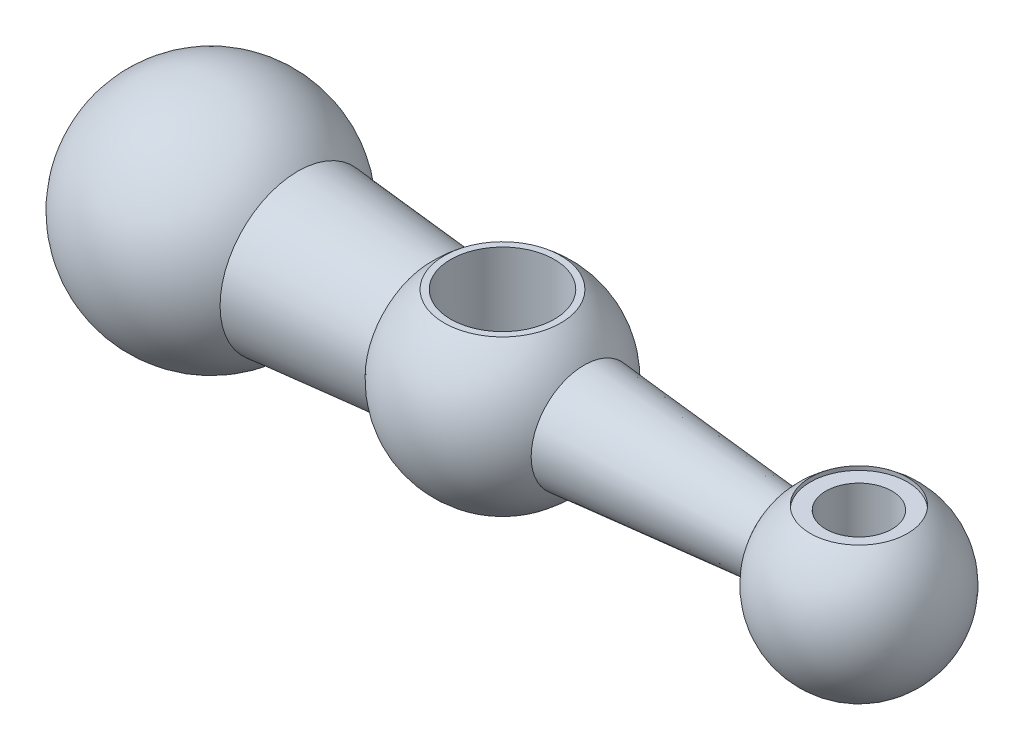
ISO-10303-21;
HEADER;
FILE_DESCRIPTION(('STEP AP214'),'2;1');
FILE_NAME('part.step','',(''),(''),'','','');
FILE_SCHEMA(('AUTOMOTIVE_DESIGN { 1 0 10303 214 1 1 1 1 }'));
ENDSEC;
DATA;
#1=APPLICATION_CONTEXT('core data for automotive mechanical design processes');
#2=APPLICATION_PROTOCOL_DEFINITION('international standard','automotive_design',2000,#1);
#3=PRODUCT_CONTEXT('',#1,'mechanical');
#4=PRODUCT('Part','Part','',(#3));
#5=PRODUCT_RELATED_PRODUCT_CATEGORY('part','',(#4));
#6=PRODUCT_DEFINITION_FORMATION('','',#4);
#7=PRODUCT_DEFINITION_CONTEXT('part definition',#1,'design');
#8=PRODUCT_DEFINITION('design','',#6,#7);
#9=PRODUCT_DEFINITION_SHAPE('','',#8);
#10=(LENGTH_UNIT() NAMED_UNIT(*) SI_UNIT(.MILLI.,.METRE.));
#11=(NAMED_UNIT(*) PLANE_ANGLE_UNIT() SI_UNIT($,.RADIAN.));
#12=(NAMED_UNIT(*) SI_UNIT($,.STERADIAN.) SOLID_ANGLE_UNIT());
#13=UNCERTAINTY_MEASURE_WITH_UNIT(LENGTH_MEASURE(1.E-05),#10,'distance_accuracy_value','');
#14=(GEOMETRIC_REPRESENTATION_CONTEXT(3) GLOBAL_UNCERTAINTY_ASSIGNED_CONTEXT((#13)) GLOBAL_UNIT_ASSIGNED_CONTEXT((#10,
#11,#12)) REPRESENTATION_CONTEXT('',''));
#15=CARTESIAN_POINT('',(0.,0.,0.));
#16=DIRECTION('',(0.,0.,1.));
#17=DIRECTION('',(1.,0.,0.));
#18=AXIS2_PLACEMENT_3D('',#15,#16,#17);
#19=CARTESIAN_POINT('',(0.,0.,0.));
#20=DIRECTION('',(-1.,0.,0.));
#21=DIRECTION('',(0.,1.,0.));
#22=AXIS2_PLACEMENT_3D('',#19,#20,#21);
#23=SPHERICAL_SURFACE('',#22,15.);
#24=CARTESIAN_POINT('',(0.,12.,0.));
#25=DIRECTION('',(0.,1.,0.));
#26=DIRECTION('',(0.,0.,1.));
#27=AXIS2_PLACEMENT_3D('',#24,#25,#26);
#28=CIRCLE('',#27,9.);
#29=CARTESIAN_POINT('',(0.,12.,9.));
#30=VERTEX_POINT('',#29);
#31=EDGE_CURVE('E62',#30,#30,#28,.T.);
#32=ORIENTED_EDGE('',*,*,#31,.F.);
#33=EDGE_LOOP('',(#32));
#34=FACE_BOUND('',#33,.T.);
#35=CARTESIAN_POINT('',(-10.9885044719242,0.,0.));
#36=DIRECTION('',(-1.,0.,0.));
#37=DIRECTION('',(0.,0.,1.));
#38=AXIS2_PLACEMENT_3D('',#35,#36,#37);
#39=CIRCLE('',#38,10.2104245489843);
#40=CARTESIAN_POINT('',(-10.9885044719242,0.,10.2104245489843));
#41=VERTEX_POINT('',#40);
#42=EDGE_CURVE('E49',#41,#41,#39,.T.);
#43=ORIENTED_EDGE('',*,*,#42,.F.);
#44=EDGE_LOOP('',(#43));
#45=FACE_BOUND('',#44,.T.);
#46=CARTESIAN_POINT('',(12.5849496103354,0.,0.));
#47=DIRECTION('',(-1.,0.,0.));
#48=DIRECTION('',(0.,0.,1.));
#49=AXIS2_PLACEMENT_3D('',#46,#47,#48);
#50=CIRCLE('',#49,8.16204896489356);
#51=CARTESIAN_POINT('',(12.5849496103354,0.,8.16204896489356));
#52=VERTEX_POINT('',#51);
#53=EDGE_CURVE('E44',#52,#52,#50,.T.);
#54=ORIENTED_EDGE('',*,*,#53,.T.);
#55=EDGE_LOOP('',(#54));
#56=FACE_BOUND('',#55,.T.);
#57=CARTESIAN_POINT('',(0.,-12.,0.));
#58=DIRECTION('',(0.,1.,0.));
#59=DIRECTION('',(0.,0.,1.));
#60=AXIS2_PLACEMENT_3D('',#57,#58,#59);
#61=CIRCLE('',#60,9.);
#62=CARTESIAN_POINT('',(0.,-12.,9.));
#63=VERTEX_POINT('',#62);
#64=EDGE_CURVE('E61',#63,#63,#61,.T.);
#65=ORIENTED_EDGE('',*,*,#64,.T.);
#66=EDGE_LOOP('',(#65));
#67=FACE_BOUND('',#66,.T.);
#68=ADVANCED_FACE('F40',(#34,#45,#56,#67),#23,.T.);
#69=CARTESIAN_POINT('',(0.,-18.,0.));
#70=DIRECTION('',(0.,1.,0.));
#71=DIRECTION('',(0.,0.,1.));
#72=AXIS2_PLACEMENT_3D('',#69,#70,#71);
#73=CYLINDRICAL_SURFACE('',#72,8.);
#74=CARTESIAN_POINT('',(0.,12.,0.));
#75=DIRECTION('',(0.,1.,0.));
#76=DIRECTION('',(0.,0.,1.));
#77=AXIS2_PLACEMENT_3D('',#74,#75,#76);
#78=CIRCLE('',#77,8.);
#79=CARTESIAN_POINT('',(0.,12.,8.));
#80=VERTEX_POINT('',#79);
#81=EDGE_CURVE('E56',#80,#80,#78,.F.);
#82=ORIENTED_EDGE('',*,*,#81,.F.);
#83=EDGE_LOOP('',(#82));
#84=FACE_BOUND('',#83,.T.);
#85=CARTESIAN_POINT('',(0.,-12.,0.));
#86=DIRECTION('',(0.,-1.,0.));
#87=DIRECTION('',(0.,0.,-1.));
#88=AXIS2_PLACEMENT_3D('',#85,#86,#87);
#89=CIRCLE('',#88,8.);
#90=CARTESIAN_POINT('',(0.,-12.,-8.));
#91=VERTEX_POINT('',#90);
#92=EDGE_CURVE('E65',#91,#91,#89,.F.);
#93=ORIENTED_EDGE('',*,*,#92,.F.);
#94=EDGE_LOOP('',(#93));
#95=FACE_BOUND('',#94,.T.);
#96=ADVANCED_FACE('F90',(#84,#95),#73,.F.);
#97=CARTESIAN_POINT('',(55.,0.,0.));
#98=DIRECTION('',(-1.,0.,0.));
#99=DIRECTION('',(0.,1.,0.));
#100=AXIS2_PLACEMENT_3D('',#97,#98,#99);
#101=SPHERICAL_SURFACE('',#100,13.);
#102=CARTESIAN_POINT('',(55.,-11.9578426147863,0.));
#103=DIRECTION('',(0.,1.,0.));
#104=DIRECTION('',(0.,0.,1.));
#105=AXIS2_PLACEMENT_3D('',#102,#103,#104);
#106=CIRCLE('',#105,5.09999999999999);
#107=CARTESIAN_POINT('',(55.,-11.9578426147863,5.09999999999999));
#108=VERTEX_POINT('',#107);
#109=EDGE_CURVE('E66',#108,#108,#106,.T.);
#110=ORIENTED_EDGE('',*,*,#109,.T.);
#111=EDGE_LOOP('',(#110));
#112=FACE_BOUND('',#111,.T.);
#113=CARTESIAN_POINT('',(43.2207810106103,0.,0.));
#114=DIRECTION('',(-1.,0.,0.));
#115=DIRECTION('',(0.,0.,1.));
#116=AXIS2_PLACEMENT_3D('',#113,#114,#115);
#117=CIRCLE('',#116,5.5);
#118=CARTESIAN_POINT('',(43.2207810106103,0.,5.5));
#119=VERTEX_POINT('',#118);
#120=EDGE_CURVE('E10',#119,#119,#117,.T.);
#121=ORIENTED_EDGE('',*,*,#120,.F.);
#122=EDGE_LOOP('',(#121));
#123=FACE_BOUND('',#122,.T.);
#124=CARTESIAN_POINT('',(55.,10.6183802907977,0.));
#125=DIRECTION('',(0.,-1.,0.));
#126=DIRECTION('',(0.,0.,-1.));
#127=AXIS2_PLACEMENT_3D('',#124,#125,#126);
#128=CIRCLE('',#127,7.49999999999999);
#129=CARTESIAN_POINT('',(55.,10.6183802907977,-7.49999999999999));
#130=VERTEX_POINT('',#129);
#131=EDGE_CURVE('E53',#130,#130,#128,.F.);
#132=ORIENTED_EDGE('',*,*,#131,.F.);
#133=EDGE_LOOP('',(#132));
#134=FACE_BOUND('',#133,.T.);
#135=ADVANCED_FACE('F39',(#112,#123,#134),#101,.T.);
#136=CARTESIAN_POINT('',(43.2207810106103,0.,0.));
#137=DIRECTION('',(-1.,0.,0.));
#138=DIRECTION('',(0.,0.,1.));
#139=AXIS2_PLACEMENT_3D('',#136,#137,#138);
#140=CONICAL_SURFACE('',#139,5.5,0.0866756064841487);
#141=ORIENTED_EDGE('',*,*,#53,.F.);
#142=EDGE_LOOP('',(#141));
#143=FACE_BOUND('',#142,.T.);
#144=ORIENTED_EDGE('',*,*,#120,.T.);
#145=EDGE_LOOP('',(#144));
#146=FACE_BOUND('',#145,.T.);
#147=ADVANCED_FACE('F92',(#143,#146),#140,.T.);
#148=CARTESIAN_POINT('',(-10.9885044719242,0.,0.));
#149=DIRECTION('',(-1.,0.,0.));
#150=DIRECTION('',(0.,0.,1.));
#151=AXIS2_PLACEMENT_3D('',#148,#149,#150);
#152=CONICAL_SURFACE('',#151,10.2104245489843,0.0866756064841487);
#153=CARTESIAN_POINT('',(-31.5835921350013,0.,0.));
#154=DIRECTION('',(-1.,0.,0.));
#155=DIRECTION('',(0.,0.,1.));
#156=AXIS2_PLACEMENT_3D('',#153,#154,#155);
#157=CIRCLE('',#156,12.);
#158=CARTESIAN_POINT('',(-31.5835921350013,0.,12.));
#159=VERTEX_POINT('',#158);
#160=EDGE_CURVE('E60',#159,#159,#157,.T.);
#161=ORIENTED_EDGE('',*,*,#160,.F.);
#162=EDGE_LOOP('',(#161));
#163=FACE_BOUND('',#162,.T.);
#164=ORIENTED_EDGE('',*,*,#42,.T.);
#165=EDGE_LOOP('',(#164));
#166=FACE_BOUND('',#165,.T.);
#167=ADVANCED_FACE('F84',(#163,#166),#152,.T.);
#168=CARTESIAN_POINT('',(-45.,0.,0.));
#169=DIRECTION('',(-1.,0.,0.));
#170=DIRECTION('',(0.,1.,0.));
#171=AXIS2_PLACEMENT_3D('',#168,#169,#170);
#172=SPHERICAL_SURFACE('',#171,18.);
#173=ORIENTED_EDGE('',*,*,#160,.T.);
#174=EDGE_LOOP('',(#173));
#175=FACE_BOUND('',#174,.T.);
#176=ADVANCED_FACE('F97',(#175),#172,.T.);
#177=CARTESIAN_POINT('',(55.,18.,0.));
#178=DIRECTION('',(0.,-1.,0.));
#179=DIRECTION('',(0.,0.,-1.));
#180=AXIS2_PLACEMENT_3D('',#177,#178,#179);
#181=CYLINDRICAL_SURFACE('',#180,7.49999999999999);
#182=CARTESIAN_POINT('',(55.,10.,0.));
#183=DIRECTION('',(0.,1.,0.));
#184=DIRECTION('',(0.,0.,1.));
#185=AXIS2_PLACEMENT_3D('',#182,#183,#184);
#186=CIRCLE('',#185,7.49999999999999);
#187=CARTESIAN_POINT('',(55.,10.,7.49999999999999));
#188=VERTEX_POINT('',#187);
#189=EDGE_CURVE('E59',#188,#188,#186,.T.);
#190=ORIENTED_EDGE('',*,*,#189,.F.);
#191=EDGE_LOOP('',(#190));
#192=FACE_BOUND('',#191,.T.);
#193=ORIENTED_EDGE('',*,*,#131,.T.);
#194=EDGE_LOOP('',(#193));
#195=FACE_BOUND('',#194,.T.);
#196=ADVANCED_FACE('F102',(#192,#195),#181,.F.);
#197=CARTESIAN_POINT('',(55.,10.,0.));
#198=DIRECTION('',(0.,1.,0.));
#199=DIRECTION('',(0.,0.,1.));
#200=AXIS2_PLACEMENT_3D('',#197,#198,#199);
#201=PLANE('',#200);
#202=CARTESIAN_POINT('',(55.,10.,0.));
#203=DIRECTION('',(0.,1.,0.));
#204=DIRECTION('',(0.,0.,1.));
#205=AXIS2_PLACEMENT_3D('',#202,#203,#204);
#206=CIRCLE('',#205,5.09999999999999);
#207=CARTESIAN_POINT('',(55.,10.,5.09999999999999));
#208=VERTEX_POINT('',#207);
#209=EDGE_CURVE('E41',#208,#208,#206,.T.);
#210=ORIENTED_EDGE('',*,*,#209,.F.);
#211=EDGE_LOOP('',(#210));
#212=FACE_BOUND('',#211,.T.);
#213=ORIENTED_EDGE('',*,*,#189,.T.);
#214=EDGE_LOOP('',(#213));
#215=FACE_BOUND('',#214,.T.);
#216=ADVANCED_FACE('F115',(#212,#215),#201,.T.);
#217=CARTESIAN_POINT('',(0.,12.,0.));
#218=DIRECTION('',(0.,1.,0.));
#219=DIRECTION('',(0.,0.,1.));
#220=AXIS2_PLACEMENT_3D('',#217,#218,#219);
#221=PLANE('',#220);
#222=ORIENTED_EDGE('',*,*,#31,.T.);
#223=EDGE_LOOP('',(#222));
#224=FACE_BOUND('',#223,.T.);
#225=ORIENTED_EDGE('',*,*,#81,.T.);
#226=EDGE_LOOP('',(#225));
#227=FACE_BOUND('',#226,.T.);
#228=ADVANCED_FACE('F116',(#224,#227),#221,.T.);
#229=CARTESIAN_POINT('',(0.,-12.,0.));
#230=DIRECTION('',(0.,-1.,0.));
#231=DIRECTION('',(0.,0.,1.));
#232=AXIS2_PLACEMENT_3D('',#229,#230,#231);
#233=PLANE('',#232);
#234=ORIENTED_EDGE('',*,*,#64,.F.);
#235=EDGE_LOOP('',(#234));
#236=FACE_BOUND('',#235,.T.);
#237=ORIENTED_EDGE('',*,*,#92,.T.);
#238=EDGE_LOOP('',(#237));
#239=FACE_BOUND('',#238,.T.);
#240=ADVANCED_FACE('F119',(#236,#239),#233,.T.);
#241=CARTESIAN_POINT('',(55.,-18.,0.));
#242=DIRECTION('',(0.,1.,0.));
#243=DIRECTION('',(0.,0.,1.));
#244=AXIS2_PLACEMENT_3D('',#241,#242,#243);
#245=CYLINDRICAL_SURFACE('',#244,5.09999999999999);
#246=ORIENTED_EDGE('',*,*,#209,.T.);
#247=EDGE_LOOP('',(#246));
#248=FACE_BOUND('',#247,.T.);
#249=ORIENTED_EDGE('',*,*,#109,.F.);
#250=EDGE_LOOP('',(#249));
#251=FACE_BOUND('',#250,.T.);
#252=ADVANCED_FACE('F121',(#248,#251),#245,.F.);
#253=CLOSED_SHELL('',(#68,#96,#135,#147,#167,#176,#196,#216,#228,#240,#252));
#254=MANIFOLD_SOLID_BREP('B2',#253);
#255=ADVANCED_BREP_SHAPE_REPRESENTATION('',(#18,#254),#14);
#256=SHAPE_DEFINITION_REPRESENTATION(#9,#255);
ENDSEC;
END-ISO-10303-21;
